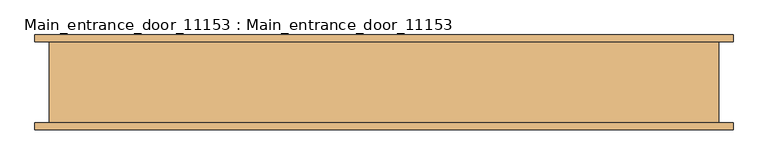
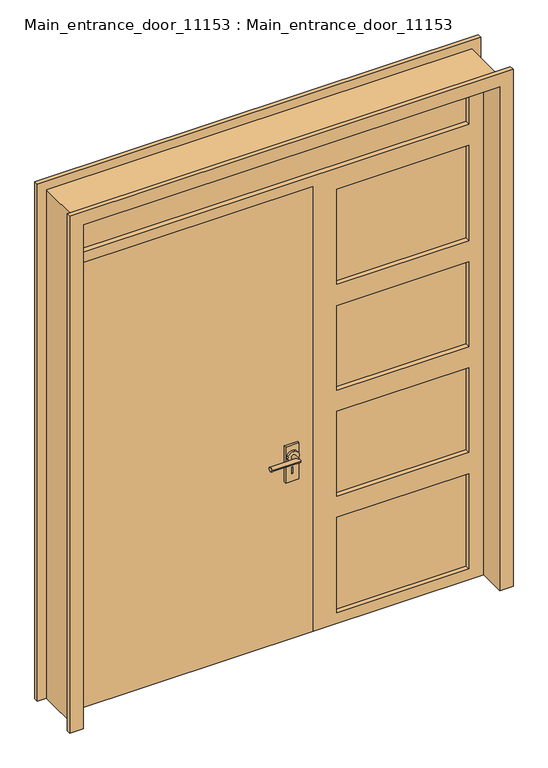
"""IFC4 building model written with IfcOpenShell, lengths in millimetres: door geometry, Main_entrance_door_11153 : Main_entrance_door_11153."""

from ifc_helpers import new_model, si_unit, point, frame, frame_2d, origin, origin_with_axes, place, context, project, spatial, polyline, circle_curve, ellipse_curve, trimmed, segment, composite_curve, outline, extrude, faceted_brep, source, transform, mapped, element, save
from ifc_brep_helpers import plane_surface, cylinder_surface, advanced_brep


def main_entrance_door_11153_main_entrance_door_11153_94c2f9e1(model_context):
    return source(origin(), model_context, "Body", "SolidModel", [
        advanced_brep(
        [(60.0, 60.0, 870.0), (80.0, 60.0, 870.0), (80.0, 100.0, 870.0), (60.0, 80.0, 870.0), (-50.0, 80.0, 870.0), (-50.0, 100.0, 870.0)],
        [
            (0, 1, circle_curve(frame((70.0, 60.0, 870.0), z_axis=(0.0, -1.0, 0.0), x_axis=(1.0, 0.0, 0.0)), 10.0)),
            (1, 0, circle_curve(frame((70.0, 60.0, 870.0), z_axis=(0.0, -1.0, 0.0), x_axis=(1.0, 0.0, 0.0)), 10.0)),
            (1, 2),
            (2, 3, ellipse_curve(frame((70.0, 90.0, 870.0), z_axis=(0.7071067811865411, -0.7071067811865538, 0.0), x_axis=(-0.7071067811865538, -0.7071067811865412, 0.0)), 14.1421356, 10.0)),
            (3, 0),
            (3, 2, ellipse_curve(frame((70.0, 90.0, 870.0), z_axis=(0.7071067811865411, -0.7071067811865538, 0.0), x_axis=(-0.7071067811865538, -0.7071067811865412, 0.0)), 14.1421356, 10.0)),
            (4, 5, circle_curve(frame((-50.0, 90.0, 870.0), z_axis=(-1.0, 0.0, 0.0), x_axis=(0.0, 1.0, 0.0)), 10.0)),
            (5, 4, circle_curve(frame((-50.0, 90.0, 870.0), z_axis=(-1.0, 0.0, 0.0), x_axis=(0.0, 1.0, 0.0)), 10.0)),
            (2, 5),
            (4, 3),
        ],
        [
            plane_surface(frame((70.0, 60.0, 870.0), z_axis=(0.0, -1.0, 0.0), x_axis=(0.0, 0.0, 1.0))),
            cylinder_surface(frame((70.0, 60.0, 870.0), z_axis=(0.0, -1.0, 0.0), x_axis=(1.0, 0.0, 0.0)), 10.0),
            plane_surface(frame((-50.0, 90.0, 870.0), z_axis=(-1.0, 0.0, 0.0), x_axis=(0.0, 0.0, 1.0))),
            cylinder_surface(frame((70.0, 90.0, 870.0), z_axis=(1.0, 0.0, 0.0), x_axis=(0.0, 1.0, 0.0)), 10.0),
        ],
        [
            (0, [[1, 2]]),
            (1, [[3, 4, 5, -2]]),
            (1, [[-5, 6, -3, -1]]),
            (2, [[7, 8]]),
            (3, [[9, -7, 10, -4]]),
            (3, [[-10, -8, -9, -6]]),
        ],
    ),
        extrude(outline(polyline([(920.0, 100.0), (920.0, 40.0), (750.0, 40.0), (750.0, 100.0), (920.0, 100.0)]), holes=[polyline([(815.3510082, 71.5671262), (785.3510082, 71.5671262), (785.3510082, 68.4328738), (815.3510082, 68.4328738), (815.3510082, 71.5671262)])]), frame((0.0, 40.0, 0.0), z_axis=(0.0, 1.0, 0.0), x_axis=(0.0, 0.0, 1.0)), (0.0, 0.0, 1.0), 10.0),
        extrude(outline(composite_curve([segment(trimmed(circle_curve(frame_2d((870.0, 70.0)), 25.0), [point((870.0, 45.0))], [point((870.0, 95.0))], False, "CARTESIAN"), True, "CONTINUOUS"), segment(trimmed(circle_curve(frame_2d((870.0, 70.0)), 25.0), [point((870.0, 95.0))], [point((870.0, 45.0))], False, "CARTESIAN"), True, "CONTINUOUS")], self_intersect=False)), frame((0.0, 40.0, 0.0), z_axis=(0.0, 1.0, 0.0), x_axis=(0.0, 0.0, 1.0)), (0.0, 0.0, 1.0), 20.0),
        advanced_brep(
        [(60.0, -30.0, 870.0), (80.0, -30.0, 870.0), (60.0, -50.0, 870.0), (80.0, -70.0, 870.0), (-50.0, -50.0, 870.0), (-50.0, -70.0, 870.0)],
        [
            (0, 1, circle_curve(frame((70.0, -30.0, 870.0), z_axis=(0.0, 1.0, 0.0), x_axis=(1.0, 0.0, 0.0)), 10.0)),
            (1, 0, circle_curve(frame((70.0, -30.0, 870.0), z_axis=(0.0, 1.0, 0.0), x_axis=(1.0, 0.0, 0.0)), 10.0)),
            (0, 2),
            (2, 3, ellipse_curve(frame((70.0, -60.0, 870.0), z_axis=(0.7071067811865457, 0.7071067811865492, 0.0), x_axis=(-0.7071067811865492, 0.7071067811865458, 0.0)), 14.1421356, 10.0)),
            (3, 1),
            (3, 2, ellipse_curve(frame((70.0, -60.0, 870.0), z_axis=(0.7071067811865457, 0.7071067811865492, 0.0), x_axis=(-0.7071067811865492, 0.7071067811865458, 0.0)), 14.1421356, 10.0)),
            (4, 5, circle_curve(frame((-50.0, -60.0, 870.0), z_axis=(-1.0, 0.0, 0.0), x_axis=(0.0, -1.0, 0.0)), 10.0)),
            (5, 4, circle_curve(frame((-50.0, -60.0, 870.0), z_axis=(-1.0, 0.0, 0.0), x_axis=(0.0, -1.0, 0.0)), 10.0)),
            (2, 4),
            (5, 3),
        ],
        [
            plane_surface(frame((70.0, -30.0, 870.0), z_axis=(0.0, 1.0, 0.0), x_axis=(0.0, 0.0, 1.0))),
            cylinder_surface(frame((70.0, -30.0, 870.0), z_axis=(0.0, 1.0, 0.0), x_axis=(1.0, 0.0, 0.0)), 10.0),
            plane_surface(frame((-50.0, -60.0, 870.0), z_axis=(-1.0, 0.0, 0.0), x_axis=(0.0, 0.0, 1.0))),
            cylinder_surface(frame((70.0, -60.0, 870.0), z_axis=(1.0, 0.0, 0.0), x_axis=(0.0, -1.0, 0.0)), 10.0),
        ],
        [
            (0, [[1, 2]]),
            (1, [[-1, 3, 4, 5]]),
            (1, [[-2, -5, 6, -3]]),
            (2, [[7, 8]]),
            (3, [[-4, 9, -8, 10]]),
            (3, [[-6, -10, -7, -9]]),
        ],
    ),
        extrude(outline(polyline([(920.0, 100.0), (920.0, 40.0), (750.0, 40.0), (750.0, 100.0), (920.0, 100.0)]), holes=[polyline([(815.3510082, 71.5671262), (785.3510082, 71.5671262), (785.3510082, 68.4328738), (815.3510082, 68.4328738), (815.3510082, 71.5671262)])]), frame((0.0, -20.0, 0.0), z_axis=(0.0, 1.0, 0.0), x_axis=(0.0, 0.0, 1.0)), (0.0, 0.0, 1.0), 10.0),
        extrude(outline(composite_curve([segment(trimmed(circle_curve(frame_2d((870.0, 70.0)), 25.0), [point((870.0, 45.0))], [point((870.0, 95.0))], False, "CARTESIAN"), True, "CONTINUOUS"), segment(trimmed(circle_curve(frame_2d((870.0, 70.0)), 25.0), [point((870.0, 95.0))], [point((870.0, 45.0))], False, "CARTESIAN"), True, "CONTINUOUS")], self_intersect=False)), frame((0.0, -30.0, 0.0), z_axis=(0.0, 1.0, 0.0), x_axis=(0.0, 0.0, 1.0)), (0.0, 0.0, 1.0), 20.0),
        faceted_brep([(990.0, 114.3, 0.0), (950.0, 114.3, 0.0), (950.0, -114.3, 0.0), (990.0, -114.3, 0.0), (990.0, -134.3, 0.0), (930.0, -134.3, 0.0), (930.0, 40.0, 0.0), (915.0, 40.0, 0.0), (915.0, 55.0, 0.0), (930.0, 55.0, 0.0), (930.0, 134.3, 0.0), (990.0, 134.3, 0.0), (990.0, 114.3, 2440.0), (-990.0, 114.3, 2440.0), (-990.0, 114.3, 0.0), (-950.0, 114.3, 0.0), (-950.0, 114.3, 2400.0), (950.0, 114.3, 2400.0), (950.0, -114.3, 2400.0), (-950.0, -114.3, 2400.0), (-950.0, -114.3, 0.0), (-990.0, -114.3, 0.0), (-990.0, -114.3, 2440.0), (990.0, -114.3, 2440.0), (990.0, -134.3, 2440.0), (-990.0, -134.3, 2440.0), (-990.0, -134.3, 0.0), (-930.0, -134.3, 0.0), (-930.0, -134.3, 2380.0), (930.0, -134.3, 2380.0), (930.0, 40.0, 2380.0), (-930.0, 40.0, 2380.0), (-930.0, 40.0, 0.0), (-915.0, 40.0, 0.0), (-915.0, 40.0, 2365.0), (915.0, 40.0, 2365.0), (915.0, 55.0, 2365.0), (-915.0, 55.0, 2365.0), (-915.0, 55.0, 0.0), (-930.0, 55.0, 0.0), (-930.0, 55.0, 2380.0), (930.0, 55.0, 2380.0), (930.0, 134.3, 2380.0), (-930.0, 134.3, 2380.0), (-930.0, 134.3, 0.0), (-990.0, 134.3, 0.0), (-990.0, 134.3, 2440.0), (990.0, 134.3, 2440.0)], [[[0, 1, 2, 3, 4, 5, 6, 7, 8, 9, 10, 11]], [[1, 0, 12, 13, 14, 15, 16, 17]], [[2, 1, 17, 18]], [[3, 2, 18, 19, 20, 21, 22, 23]], [[4, 3, 23, 24]], [[5, 4, 24, 25, 26, 27, 28, 29]], [[6, 5, 29, 30]], [[7, 6, 30, 31, 32, 33, 34, 35]], [[8, 7, 35, 36]], [[9, 8, 36, 37, 38, 39, 40, 41]], [[10, 9, 41, 42]], [[11, 10, 42, 43, 44, 45, 46, 47]], [[0, 11, 47, 12]], [[14, 13, 46, 45]], [[15, 14, 45, 44, 39, 38, 33, 32, 27, 26, 21, 20]], [[16, 15, 20, 19]], [[22, 21, 26, 25]], [[28, 27, 32, 31]], [[34, 33, 38, 37]], [[40, 39, 44, 43]], [[13, 12, 47, 46]], [[17, 16, 19, 18]], [[23, 22, 25, 24]], [[29, 28, 31, 30]], [[35, 34, 37, 36]], [[41, 40, 43, 42]]]),
        faceted_brep([(225.0, 40.0, 0.0), (930.0, 40.0, 0.0), (930.0, -10.0, 0.0), (170.0, -10.0, 0.0), (170.0, 40.0, 0.0), (155.0, 40.0, 0.0), (155.0, 55.0, 0.0), (225.0, 55.0, 0.0), (225.0, 40.0, 2100.0), (930.0, 40.0, 2100.0), (865.0, 40.0, 500.0), (275.0, 40.0, 500.0), (275.0, 40.0, 50.0), (865.0, 40.0, 50.0), (865.0, 40.0, 1000.0), (275.0, 40.0, 1000.0), (275.0, 40.0, 600.0), (865.0, 40.0, 600.0), (865.0, 40.0, 1500.0), (275.0, 40.0, 1500.0), (275.0, 40.0, 1100.0), (865.0, 40.0, 1100.0), (865.0, 40.0, 2050.0), (275.0, 40.0, 2050.0), (275.0, 40.0, 1600.0), (865.0, 40.0, 1600.0), (930.0, 55.0, 2100.0), (930.0, 55.0, 2380.0), (930.0, -10.0, 2380.0), (-930.0, -10.0, 2380.0), (-930.0, -10.0, 2100.0), (170.0, -10.0, 2100.0), (275.0, -10.0, 500.0), (865.0, -10.0, 500.0), (865.0, -10.0, 50.0), (275.0, -10.0, 50.0), (275.0, -10.0, 1000.0), (865.0, -10.0, 1000.0), (865.0, -10.0, 600.0), (275.0, -10.0, 600.0), (-880.0, -10.0, 2315.0), (865.0, -10.0, 2315.0), (865.0, -10.0, 2150.0), (-880.0, -10.0, 2150.0), (275.0, -10.0, 1500.0), (865.0, -10.0, 1500.0), (865.0, -10.0, 1100.0), (275.0, -10.0, 1100.0), (275.0, -10.0, 2050.0), (865.0, -10.0, 2050.0), (865.0, -10.0, 1600.0), (275.0, -10.0, 1600.0), (170.0, 40.0, 2100.0), (155.0, 40.0, 2100.0), (155.0, 55.0, 2100.0), (-930.0, 55.0, 2100.0), (-930.0, 55.0, 2380.0), (225.0, 55.0, 2100.0), (865.0, 55.0, 2315.0), (-880.0, 55.0, 2315.0), (-880.0, 55.0, 2150.0), (865.0, 55.0, 2150.0)], [[[0, 1, 2, 3, 4, 5, 6, 7]], [[1, 0, 8, 9], [10, 11, 12, 13], [14, 15, 16, 17], [18, 19, 20, 21], [22, 23, 24, 25]], [[2, 1, 9, 26, 27, 28]], [[3, 2, 28, 29, 30, 31], [32, 33, 34, 35], [36, 37, 38, 39], [40, 41, 42, 43], [44, 45, 46, 47], [48, 49, 50, 51]], [[4, 3, 31, 52]], [[5, 4, 52, 53]], [[6, 5, 53, 54]], [[7, 6, 54, 55, 56, 27, 26, 57], [58, 59, 60, 61]], [[0, 7, 57, 8]], [[10, 33, 32, 11]], [[33, 10, 13, 34]], [[12, 35, 34, 13]], [[11, 32, 35, 12]], [[14, 37, 36, 15]], [[37, 14, 17, 38]], [[16, 39, 38, 17]], [[15, 36, 39, 16]], [[45, 18, 21, 46]], [[20, 47, 46, 21]], [[19, 44, 47, 20]], [[27, 56, 29, 28]], [[29, 56, 55, 30]], [[58, 41, 40, 59]], [[41, 58, 61, 42]], [[59, 40, 43, 60]], [[18, 45, 44, 19]], [[22, 49, 48, 23]], [[24, 51, 50, 25]], [[23, 48, 51, 24]], [[49, 22, 25, 50]], [[57, 26, 9, 8]], [[30, 55, 54, 53, 52, 31]], [[60, 43, 42, 61]]]),
        extrude(outline(polyline([(170.0, 40.0), (170.0, -10.0), (-930.0, -10.0), (-930.0, 40.0), (170.0, 40.0)])), origin_with_axes(), (0.0, 0.0, 1.0), 2100.0),
        extrude(outline(polyline([(-880.0, 12.0), (-880.0, 18.0), (865.0, 18.0), (865.0, 12.0), (-880.0, 12.0)])), frame((0.0, 0.0, 2150.0), z_axis=(0.0, 0.0, 1.0), x_axis=(1.0, 0.0, 0.0)), (0.0, 0.0, 1.0), 165.0),
        extrude(outline(polyline([(865.0, 18.0), (865.0, 12.0), (275.0, 12.0), (275.0, 18.0), (865.0, 18.0)])), frame((0.0, 0.0, 50.0), z_axis=(0.0, 0.0, 1.0), x_axis=(1.0, 0.0, 0.0)), (0.0, 0.0, 1.0), 450.0),
        extrude(outline(polyline([(865.0, 18.0), (865.0, 12.0), (275.0, 12.0), (275.0, 18.0), (865.0, 18.0)])), frame((0.0, 0.0, 600.0), z_axis=(0.0, 0.0, 1.0), x_axis=(1.0, 0.0, 0.0)), (0.0, 0.0, 1.0), 400.0),
        extrude(outline(polyline([(865.0, 18.0), (865.0, 12.0), (275.0, 12.0), (275.0, 18.0), (865.0, 18.0)])), frame((0.0, 0.0, 1600.0), z_axis=(0.0, 0.0, 1.0), x_axis=(1.0, 0.0, 0.0)), (0.0, 0.0, 1.0), 450.0),
        extrude(outline(polyline([(865.0, 18.0), (865.0, 12.0), (275.0, 12.0), (275.0, 18.0), (865.0, 18.0)])), frame((0.0, 0.0, 1100.0), z_axis=(0.0, 0.0, 1.0), x_axis=(1.0, 0.0, 0.0)), (0.0, 0.0, 1.0), 400.0),
    ])


if __name__ == "__main__":
    model = new_model("IFC4")
    model_context = context("Model", 3, world=origin())
    ifc_project = project(units=[si_unit("LENGTHUNIT", "METRE", prefix="MILLI")], contexts=[model_context])
    site = spatial("IfcSite", under=ifc_project)
    building = spatial("IfcBuilding", under=site)
    placement = place(None, origin())
    main_entrance_door_11153_main_entrance_door_11153_shape = main_entrance_door_11153_main_entrance_door_11153_94c2f9e1(model_context)
    element("IfcDoor", 1, ObjectType="Main_entrance_door_11153 : Main_entrance_door_11153", at=placement, inside=building, context=model_context, shape_type="MappedRepresentation", body=[
        mapped(main_entrance_door_11153_main_entrance_door_11153_shape, transform((0.0, 0.0, 0.0), x_axis=(1.0, 0.0, 0.0), y_axis=(0.0, 1.0, 0.0), z_axis=(0.0, 0.0, 1.0))),
    ])
    save(model, "model.ifc")

# Revit data of these elements
# Type "Main_entrance_door_11153 : Main_entrance_door_11153"
#   Type Mark = "8"
#   Height = 7' - 10.48819"
#   Width = 6' - 2.80315"
#   Door Width = 3' - 7.30709"
#   Function = (empty or 0)
#   Wall Closure = (empty or 0)
# Element 1 (IfcDoor, "Main_entrance_door_11153 : Main_entrance_door_11153")
#   Materials on its faces: "Glass", "Default"
# Materials
#   "Glass": class "Glass", colour RGB 0 128 192, transparency 0.75, Description = "Soda Lime Glass", Cost = 0
#   "Default": colour RGB 127 127 127, transparency 0, Cost = 0
